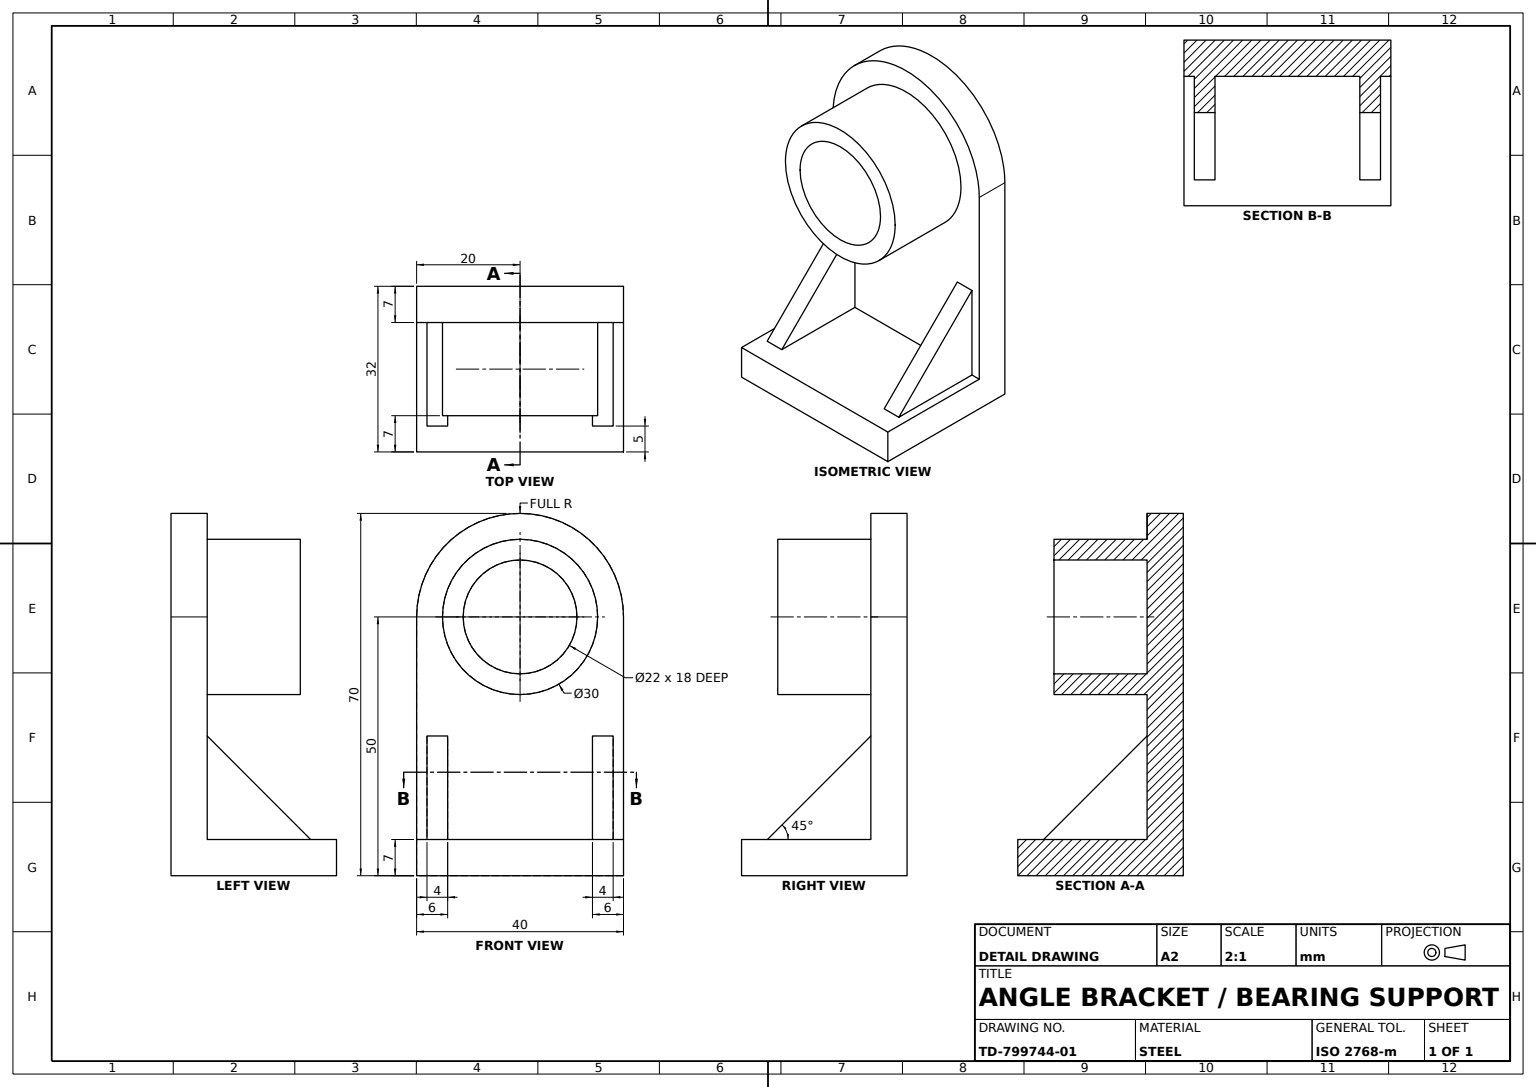
from build123d import *

# Parameters (mm, degrees)
BASE_ANGLE_DEPTH             = 20
UPRIGHT_PLATE_SKETCH_W       = 40
UPRIGHT_PLATE_SKETCH_H       = 43
UPRIGHT_PLATE_DEPTH          = 7
BEARING_HUB_SKETCH_R         = 15
BEARING_HUB_SKETCH_R_2       = 11
BEARING_HUB_30_BORE_22_DEPTH = 18
GUSSET_START                 = -6
GUSSET_RIB_DEPTH             = 4


with BuildPart() as part:
    # Base Angle Profile Sketch → Base Angle (new, symmetric)
    with BuildSketch(Plane(origin=(0, 0, 0), x_dir=(0, 0, -1), z_dir=(1, 0, 0))):
        Polygon((0, 0), (32, 0), (32, 50), (25, 50), (25, 7), (0, 7), align=None)
    extrude(amount=BASE_ANGLE_DEPTH, both=True)

    # Upright Plate Sketch → Upright Plate (add)
    with BuildSketch(Plane.XY.offset(-25)):
        with Locations((0, 28.5)):
            Rectangle(UPRIGHT_PLATE_SKETCH_W, UPRIGHT_PLATE_SKETCH_H)
        with BuildLine():
            ThreePointArc((20, 50), (0, 70), (-20, 50))
            Line((-20, 50), (20, 50))
        make_face()
    extrude(amount=-UPRIGHT_PLATE_DEPTH)

    # Bearing Hub Sketch → Bearing Hub Ø30 Bore Ø22 (add)
    with BuildSketch(Plane.XY.offset(-25)):
        with Locations(Location((0, 50, 0), (0, 0, 90))):
            Circle(BEARING_HUB_SKETCH_R)
        with Locations((0, 50)):
            Circle(BEARING_HUB_SKETCH_R_2, mode=Mode.SUBTRACT)
    extrude(amount=BEARING_HUB_30_BORE_22_DEPTH)

    # Gusset Rib Sketch → Gusset Rib (add)
    with BuildSketch(Plane(origin=(20, 0, 0), x_dir=(0, 0, -1), z_dir=(1, 0, 0)).offset(GUSSET_START)):
        Polygon((5, 7), (25, 27), (25, 7), align=None)
    gusset_rib = extrude(amount=GUSSET_RIB_DEPTH)

    # Gusset Rib Mirror: Gusset Rib across plane
    add(gusset_rib.mirror(Plane(origin=(0, 0, 0), x_dir=(0, 0, 1), z_dir=(1, 0, 0))))


solid = part.part
